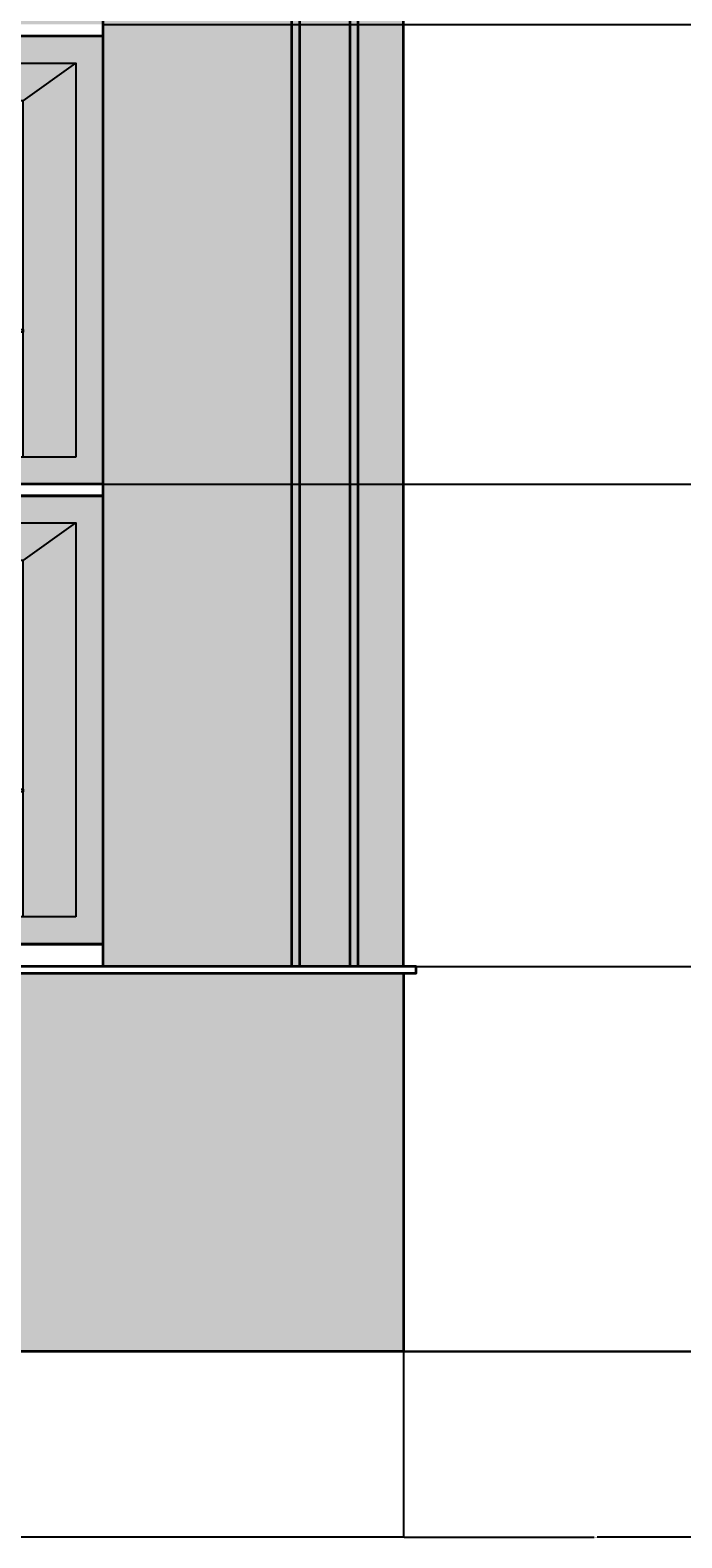
# Model space of a CAD drawing. Units: feet. Extents: x 1141 to 2858, y 751 to 1654.
# Tile 4 of 13: x 2096 to 2288, y 751 to 1195. Entities that reach past the tile are written whole.
import ezdxf

# ---------------------------------------------------------------- set-up
doc = ezdxf.new("R2010")
doc.units = ezdxf.units.FT
for name, color, linetype, lineweight in [('A-ANNO-DIMS', 2, 'Continuous', 18), ('A-ELEV', 7, 'Continuous', 35), ('A-ELEV-PATT', 8, 'Continuous', 13), ('A-GLAZ', 4, 'Continuous', 25)]:
    doc.layers.add(name, color=color, linetype=linetype, lineweight=lineweight)
doc.styles.get("Standard").update_dxf_attribs({"font": 'arial.ttf'})
doc.dimstyles.get("Standard").update_dxf_attribs({"dimtxt": 0.18, "dimasz": 0.18, "dimexe": 0.18, "dimexo": 0.0625, "dimgap": 0.09, "dimtad": 0, "dimtih": 1, "dimtoh": 1, "dimdec": 1, "dimzin": 0, "dimdsep": 46, "dimlunit": 3, "dimtxsty": 'Standard', "dimcen": 0.09, "dimadec": 0, "dimazin": 0, "dimtfac": 1, "dimtdec": 1, "dimtofl": 0, "dimtmove": 0, "dimatfit": 3, "dimfxl": 1, "dimtolj": 1, "dimtzin": 0, "dimarcsym": 0})

# ---------------------------------------------------------------- blocks, each defined once
blk = doc.blocks.new('WIN-SIDE-A')
blk.add_line((63.09, 104.94), (78.57, 116.03))
blk.add_line((63.09, 104.94), (78.57, 116.03))
for points in [[(78.57, 0), (0, 0), (0, 116.03), (78.57, 116.03)], [(78.57, 0), (0, 0), (0, 116.03), (78.57, 116.03)], [(31.54, 104.94), (32.46, 104.94), (32.46, 0), (31.54, 0)], [(0, 37.61), (63.09, 37.61), (63.09, 36.79), (0, 36.79)]]:
    blk.add_lwpolyline(points, close=True)
for points in [[(63.09, 0), (63.09, 104.94), (0, 104.94)], [(63.09, 0), (63.09, 104.94), (0, 104.94)], [(31.54, 37.61), (31.54, 104.94), (32.46, 104.94), (32.46, 37.61)], [(31.54, 36.79), (0, 36.79), (0, 37.61), (31.54, 37.61)], [(32.46, 36.79), (32.46, 0), (31.54, 0), (31.54, 36.79)], [(32.46, 37.61), (63.09, 37.61), (63.09, 36.79), (32.46, 36.79)]]:
    blk.add_lwpolyline(points)
blk = doc.blocks.new('*D22')
at = {"layer": 'A-ANNO-DIMS', "color": 0, "lineweight": -2, "transparency": 16777216}
for p, q in [((1726.03, 805.84), (1726.03, 751.07)), ((2206.03, 805.84), (2206.03, 751.07)), ((1726.21, 751.25), (1965.74, 751.25)), ((2205.85, 751.25), (1966.32, 751.25))]:
    blk.add_line(p, q, dxfattribs=at)
at = {"layer": 'A-ANNO-DIMS', "color": 0, "transparency": 16777216}
for points in [[(1726.21, 751.28), (1726.21, 751.22), (1726.03, 751.25)], [(2205.85, 751.28), (2205.85, 751.22), (2206.03, 751.25)]]:
    blk.add_solid(points, dxfattribs=at)
at = {"layer": 'Defpoints', "color": 0, "transparency": 16777216}
for p in [(1726.03, 805.9), (2206.03, 805.9), (2206.03, 751.25)]:
    blk.add_point(p, dxfattribs=at)
at = {"layer": 'A-ANNO-DIMS', "color": 0, "transparency": 16777216, "insert": (1966.03, 751.25), "char_height": 0.18, "attachment_point": 5}
blk.add_mtext('\\A1;480', dxfattribs=at)
blk = doc.blocks.new('*D23')
at = {"layer": 'A-ANNO-DIMS', "color": 0, "lineweight": -2, "transparency": 16777216}
for p, q in [((2206.03, 805.84), (2206.03, 751.07)), ((2319.3, 805.84), (2319.3, 751.07)), ((2206.21, 751.25), (2262.21, 751.25)), ((2319.12, 751.25), (2263.12, 751.25))]:
    blk.add_line(p, q, dxfattribs=at)
at = {"layer": 'A-ANNO-DIMS', "color": 0, "transparency": 16777216}
for points in [[(2206.21, 751.28), (2206.21, 751.22), (2206.03, 751.25)], [(2319.12, 751.28), (2319.12, 751.22), (2319.3, 751.25)]]:
    blk.add_solid(points, dxfattribs=at)
at = {"layer": 'Defpoints', "color": 0, "transparency": 16777216}
for p in [(2206.03, 805.9), (2319.3, 805.9), (2319.3, 751.25)]:
    blk.add_point(p, dxfattribs=at)
at = {"layer": 'A-ANNO-DIMS', "color": 0, "transparency": 16777216, "insert": (2262.67, 751.25), "char_height": 0.18, "attachment_point": 5}
blk.add_mtext('\\A1;113.27', dxfattribs=at)
blk = doc.blocks.new('*D29')
at = {"layer": 'A-ANNO-DIMS', "color": 0, "lineweight": -2, "transparency": 16777216}
for p, q in [((2206.09, 919.34), (2857.83, 919.34)), ((2857.65, 919.16), (2857.65, 862.8)), ((2857.65, 806.08), (2857.65, 862.44)), ((2206.09, 805.9), (2857.83, 805.9))]:
    blk.add_line(p, q, dxfattribs=at)
at = {"layer": 'A-ANNO-DIMS', "color": 0, "transparency": 16777216}
for points in [[(2857.62, 919.16), (2857.68, 919.16), (2857.65, 919.34)], [(2857.62, 806.08), (2857.68, 806.08), (2857.65, 805.9)]]:
    blk.add_solid(points, dxfattribs=at)
at = {"layer": 'Defpoints', "color": 0, "transparency": 16777216}
for p in [(2206.03, 919.34), (2857.65, 919.34), (2206.03, 805.9)]:
    blk.add_point(p, dxfattribs=at)
at = {"layer": 'A-ANNO-DIMS', "color": 0, "transparency": 16777216, "insert": (2857.65, 862.62), "char_height": 0.18, "attachment_point": 5}
blk.add_mtext('\\A1;113.44', dxfattribs=at)
blk = doc.blocks.new('*D30')
at = {"layer": 'A-ANNO-DIMS', "color": 0, "lineweight": -2, "transparency": 16777216}
for p, q in [((2117.47, 1061.29), (2857.83, 1061.29)), ((2857.65, 1061.11), (2857.65, 990.5)), ((2857.65, 919.52), (2857.65, 990.13)), ((2117.47, 919.34), (2857.83, 919.34))]:
    blk.add_line(p, q, dxfattribs=at)
at = {"layer": 'A-ANNO-DIMS', "color": 0, "transparency": 16777216}
for points in [[(2857.62, 1061.11), (2857.68, 1061.11), (2857.65, 1061.29)], [(2857.62, 919.52), (2857.68, 919.52), (2857.65, 919.34)]]:
    blk.add_solid(points, dxfattribs=at)
at = {"layer": 'Defpoints', "color": 0, "transparency": 16777216}
for p in [(2117.41, 1061.29), (2857.65, 1061.29), (2117.41, 919.34)]:
    blk.add_point(p, dxfattribs=at)
at = {"layer": 'A-ANNO-DIMS', "color": 0, "transparency": 16777216, "insert": (2857.65, 990.31), "char_height": 0.18, "attachment_point": 5}
blk.add_mtext('\\A1;141.95', dxfattribs=at)
blk = doc.blocks.new('*D31')
at = {"layer": 'A-ANNO-DIMS', "color": 0, "lineweight": -2, "transparency": 16777216}
for p, q in [((2117.47, 1196.68), (2857.83, 1196.68)), ((2857.65, 1196.5), (2857.65, 1129.16)), ((2857.65, 1061.47), (2857.65, 1128.8)), ((2117.47, 1061.29), (2857.83, 1061.29))]:
    blk.add_line(p, q, dxfattribs=at)
at = {"layer": 'A-ANNO-DIMS', "color": 0, "transparency": 16777216}
for points in [[(2857.62, 1196.5), (2857.68, 1196.5), (2857.65, 1196.68)], [(2857.62, 1061.47), (2857.68, 1061.47), (2857.65, 1061.29)]]:
    blk.add_solid(points, dxfattribs=at)
at = {"layer": 'Defpoints', "color": 0, "transparency": 16777216}
for p in [(2117.41, 1196.68), (2857.65, 1196.68), (2117.41, 1061.29)]:
    blk.add_point(p, dxfattribs=at)
at = {"layer": 'A-ANNO-DIMS', "color": 0, "transparency": 16777216, "insert": (2857.65, 1128.98), "char_height": 0.18, "attachment_point": 5}
blk.add_mtext('\\A1;135.4', dxfattribs=at)
blk = doc.blocks.new('*D39')
at = {"layer": 'A-ANNO-DIMS', "color": 0, "lineweight": -2, "transparency": 16777216}
for p, q in [((2319.24, 1599.45), (1668.14, 1599.45)), ((1668.32, 1599.27), (1668.32, 1202.86)), ((1668.32, 806.08), (1668.32, 1202.49)), ((2319.24, 805.9), (1668.14, 805.9))]:
    blk.add_line(p, q, dxfattribs=at)
at = {"layer": 'A-ANNO-DIMS', "color": 0, "transparency": 16777216}
for points in [[(1668.29, 1599.27), (1668.35, 1599.27), (1668.32, 1599.45)], [(1668.29, 806.08), (1668.35, 806.08), (1668.32, 805.9)]]:
    blk.add_solid(points, dxfattribs=at)
at = {"layer": 'Defpoints', "color": 0, "transparency": 16777216}
for p in [(1668.32, 1599.45), (2319.3, 1599.45), (2319.3, 805.9)]:
    blk.add_point(p, dxfattribs=at)
at = {"layer": 'A-ANNO-DIMS', "color": 0, "transparency": 16777216, "insert": (1668.32, 1202.68), "char_height": 0.18, "attachment_point": 5}
blk.add_mtext('\\A1;793.6', dxfattribs=at)

msp = doc.modelspace()

# ---------------------------------------------------------------- hatches: boundary and pattern name
at = {"layer": 'A-ELEV-PATT'}
h = msp.add_hatch(color=256, dxfattribs=at)
h.dxf.hatch_style = 1
h.paths.add_polyline_path([(2206.032, 1599.4527), (2192.689, 1599.4527), (2192.689, 919.339), (2206.032, 919.339)])
h.paths.add_polyline_path([(2190.2416, 1599.4527), (2175.463, 1599.4527), (2175.463, 919.339), (2190.2416, 919.339)])
h.paths.add_polyline_path([(2173.0156, 1599.4527), (2117.407, 1599.4527), (2117.407, 919.339), (2173.0156, 919.339)])
h.paths.add_polyline_path([(2022.8666, 1057.9008), (1726.032, 1057.9008), (1726.032, 925.9008), (2022.8666, 925.9008)])
h.paths.add_polyline_path([(1737.6123, 937.4811), (1737.6123, 1046.3205), (2011.2863, 1046.3205), (2011.2863, 937.4811)], flags=16)
h.paths.add_polyline_path([(1754.2423, 946.7736), (1754.2423, 1033.2183), (2004.2323, 1033.2183), (2004.2323, 946.7736), (2004.3069, 946.6754), (1906.0824, 946.6754)], flags=0)
h.paths.add_polyline_path([(1900.5421, 946.7736), (1857.5566, 946.7736), (1857.5566, 1033.2183), (1900.5421, 1033.2183)], flags=0)
h.paths.add_polyline_path([(1910.8368, 951.4297), (1910.8368, 1022.7957), (1999.478, 1022.7957), (1999.478, 951.4297)], flags=0)
h.paths.add_polyline_path([(1930.8039, 951.4297), (1930.8039, 1022.7957), (1932.373, 1022.7957), (1932.373, 951.4297)], flags=0)
h.paths.add_polyline_path([(1851.6414, 946.7736), (1826.5664, 946.7736), (1826.5664, 967.8234), (1793.4402, 967.8234), (1793.4402, 946.7736), (1790.4043, 946.7736), (1790.4043, 967.8234), (1754.2423, 967.8234), (1754.2423, 970.4796), (1790.4043, 970.4796), (1790.4043, 1033.2183), (1793.4402, 1033.2183), (1793.4402, 970.4796), (1826.5664, 970.4796), (1826.5664, 1033.2183), (1851.6414, 1033.2183)], flags=0)
h.paths.add_polyline_path([(1954.3728, 951.4297), (1954.3728, 1022.7957), (1955.9419, 1022.7957), (1955.9419, 951.4297)], flags=0)
h.paths.add_polyline_path([(1977.7327, 951.4297), (1977.7327, 1022.7957), (1979.3018, 1022.7957), (1979.3018, 951.4297)], flags=0)
h.paths.add_polyline_path([(2022.8666, 1193.2888), (1726.032, 1193.2888), (1726.032, 1061.2888), (2022.8666, 1061.2888)])
h.paths.add_polyline_path([(1737.6123, 1072.869), (1737.6123, 1181.7085), (2011.2863, 1181.7085), (2011.2863, 1072.869)], flags=16)
h.paths.add_polyline_path([(1754.2423, 1082.1616), (1754.2423, 1168.6063), (2004.2323, 1168.6063), (2004.2323, 1082.1616), (2004.3069, 1082.0634), (1906.0824, 1082.0634)], flags=0)
h.paths.add_polyline_path([(1900.5421, 1082.1616), (1857.5566, 1082.1616), (1857.5566, 1168.6063), (1900.5421, 1168.6063)], flags=0)
h.paths.add_polyline_path([(1910.8368, 1086.8177), (1910.8368, 1158.1837), (1999.478, 1158.1837), (1999.478, 1086.8177)], flags=0)
h.paths.add_polyline_path([(1930.8039, 1086.8177), (1930.8039, 1158.1837), (1932.373, 1158.1837), (1932.373, 1086.8177)], flags=0)
h.paths.add_polyline_path([(1851.6414, 1082.1616), (1826.5664, 1082.1616), (1826.5664, 1103.2114), (1793.4402, 1103.2114), (1793.4402, 1082.1616), (1790.4043, 1082.1616), (1790.4043, 1103.2114), (1754.2423, 1103.2114), (1754.2423, 1105.8676), (1790.4043, 1105.8676), (1790.4043, 1168.6063), (1793.4402, 1168.6063), (1793.4402, 1105.8676), (1826.5664, 1105.8676), (1826.5664, 1168.6063), (1851.6414, 1168.6063)], flags=0)
h.paths.add_polyline_path([(1954.3728, 1086.8177), (1954.3728, 1158.1837), (1955.9419, 1158.1837), (1955.9419, 1086.8177)], flags=0)
h.paths.add_polyline_path([(1977.7327, 1086.8177), (1977.7327, 1158.1837), (1979.3018, 1158.1837), (1979.3018, 1086.8177)], flags=0)
h.paths.add_polyline_path([(2022.8666, 1599.4527), (1726.032, 1599.4527), (1726.032, 1467.4527), (2022.8666, 1467.4527)])
h.paths.add_polyline_path([(2011.2863, 1479.033), (1737.6123, 1479.033), (1737.6123, 1587.8725), (2011.2863, 1587.8725)], flags=16)
h.paths.add_polyline_path([(2004.2323, 1488.3255), (1754.2423, 1488.3255), (1754.2423, 1574.7702), (2004.2323, 1574.7702)], flags=0)
h.paths.add_polyline_path([(1829.1345, 1544.6458), (1914.1177, 1544.6458), (1914.1177, 1539.5463), (1830.9097, 1539.5463), (1831.6817, 1537.3286), (1914.1177, 1537.3286), (1914.1177, 1532.2291), (1833.4569, 1532.2291), (1834.229, 1530.0113), (1914.1177, 1530.0113), (1914.1177, 1524.9118), (1836.0042, 1524.9118), (1836.7762, 1522.694), (1914.1177, 1522.694), (1914.1177, 1517.5946), (1838.5514, 1517.5946), (1839.3235, 1515.3768), (1914.1177, 1515.3768), (1914.1177, 1510.2773), (1841.0987, 1510.2773), (1841.8707, 1508.0595), (1914.1177, 1508.0595), (1914.1177, 1502.9601), (1843.6459, 1502.9601), (1844.4179, 1500.7423), (1914.1177, 1500.7423), (1914.1177, 1495.6428), (1846.1931, 1495.6428), (1846.9652, 1493.425), (1914.1177, 1493.425), (1914.1177, 1488.3255), (1848.6593, 1488.3255), (1848.6593, 1488.5583)], flags=0)
h.paths.add_polyline_path([(2117.407, 1464.0647), (1820.5724, 1464.0647), (1820.5724, 1332.0647), (2117.407, 1332.0647)])
h.paths.add_polyline_path([(2105.8267, 1452.4845), (2105.8267, 1343.645), (1832.1527, 1343.645), (1832.1527, 1452.4845)], flags=16)
h.paths.add_polyline_path([(2089.1967, 1439.3822), (2089.1967, 1352.9376), (1937.3566, 1352.9376), (1937.3566, 1352.8393), (1839.1321, 1352.8393), (1839.2067, 1352.9376), (1839.2067, 1439.3822), (1937.3566, 1439.3822)], flags=0)
h.paths.add_polyline_path([(2016.8727, 1439.3822), (2016.8727, 1376.6436), (2049.9988, 1376.6436), (2049.9988, 1439.3822), (2053.0347, 1439.3822), (2053.0347, 1376.6436), (2089.1967, 1376.6436), (2089.1967, 1373.9873), (2053.0347, 1373.9873), (2053.0347, 1352.9376), (2049.9988, 1352.9376), (2049.9988, 1373.9873), (2016.8727, 1373.9873), (2016.8727, 1352.9376), (1991.7976, 1352.9376), (1991.7976, 1439.3822)], flags=0)
h.paths.add_polyline_path([(1985.8824, 1439.3822), (1985.8824, 1352.9376), (1942.8969, 1352.9376), (1942.8969, 1439.3822)], flags=0)
h.paths.add_polyline_path([(1932.6022, 1428.9596), (1932.6022, 1357.5937), (1843.961, 1357.5937), (1843.961, 1428.9596)], flags=0)
h.paths.add_polyline_path([(1912.6351, 1428.9596), (1912.6351, 1357.5937), (1911.066, 1357.5937), (1911.066, 1428.9596)], flags=0)
h.paths.add_polyline_path([(1889.0662, 1428.9596), (1889.0662, 1357.5937), (1887.4971, 1357.5937), (1887.4971, 1428.9596)], flags=0)
h.paths.add_polyline_path([(1865.7063, 1428.9596), (1865.7063, 1357.5937), (1864.1372, 1357.5937), (1864.1372, 1428.9596)], flags=0)
h.paths.add_polyline_path([(2117.407, 1328.6768), (1820.5724, 1328.6768), (1820.5724, 1196.6768), (2117.407, 1196.6768)])
h.paths.add_polyline_path([(2105.8267, 1317.0965), (2105.8267, 1208.257), (1832.1527, 1208.257), (1832.1527, 1317.0965)], flags=16)
h.paths.add_polyline_path([(2089.1967, 1303.9943), (2089.1967, 1217.5496), (1937.3566, 1217.5496), (1937.3566, 1217.4513), (1839.1321, 1217.4513), (1839.2067, 1217.5496), (1839.2067, 1303.9943), (1937.3566, 1303.9943)], flags=0)
h.paths.add_polyline_path([(2016.8727, 1303.9943), (2016.8727, 1241.2556), (2049.9988, 1241.2556), (2049.9988, 1303.9943), (2053.0347, 1303.9943), (2053.0347, 1241.2556), (2089.1967, 1241.2556), (2089.1967, 1238.5993), (2053.0347, 1238.5993), (2053.0347, 1217.5496), (2049.9988, 1217.5496), (2049.9988, 1238.5993), (2016.8727, 1238.5993), (2016.8727, 1217.5496), (1991.7976, 1217.5496), (1991.7976, 1303.9943)], flags=0)
h.paths.add_polyline_path([(1985.8824, 1303.9943), (1985.8824, 1217.5496), (1942.8969, 1217.5496), (1942.8969, 1303.9943)], flags=0)
h.paths.add_polyline_path([(1932.6022, 1293.5716), (1932.6022, 1222.2057), (1843.961, 1222.2057), (1843.961, 1293.5716)], flags=0)
h.paths.add_polyline_path([(1912.6351, 1293.5716), (1912.6351, 1222.2057), (1911.066, 1222.2057), (1911.066, 1293.5716)], flags=0)
h.paths.add_polyline_path([(1889.0662, 1293.5716), (1889.0662, 1222.2057), (1887.4971, 1222.2057), (1887.4971, 1293.5716)], flags=0)
h.paths.add_polyline_path([(1865.7063, 1293.5716), (1865.7063, 1222.2057), (1864.1372, 1222.2057), (1864.1372, 1293.5716)], flags=0)
h.paths.add_polyline_path([(2206.032, 917.3598), (2027.2589, 917.3598), (2027.2589, 805.9008), (2206.032, 805.9008)])
h.paths.add_polyline_path([(1852.1771, 917.3598), (1726.032, 917.3598), (1726.032, 805.9008), (1852.1771, 805.9008)])
h.paths.add_polyline_path([(2063.3101, 1580.3829), (2093.938, 1580.3829), (2093.938, 1513.0494), (2063.3101, 1513.0494)])
h.paths.add_polyline_path([(2063.3101, 1580.3829), (2093.938, 1580.3829), (2093.938, 1513.0494), (2063.3101, 1513.0494)])
h = msp.add_hatch(color=256, dxfattribs=at)
h.dxf.hatch_style = 1
h.paths.add_polyline_path([(2011.2863, 1587.8725), (1737.6123, 1587.8725), (1754.2423, 1574.7702), (2004.2323, 1574.7702)])
h.paths.add_polyline_path([(1754.2423, 1574.7702), (1737.6123, 1587.8725), (1737.6123, 1479.033), (1754.2423, 1488.3255)])
h.paths.add_polyline_path([(2011.2863, 1587.8725), (2004.2323, 1574.7702), (2004.2323, 1488.3255), (2011.2863, 1479.033)])
h.paths.add_polyline_path([(2004.2323, 1488.3255), (1754.2423, 1488.3255), (1737.6123, 1479.033), (2011.2863, 1479.033)])
h.paths.add_polyline_path([(2105.8267, 1452.4845), (1832.1527, 1452.4845), (1839.2067, 1439.3822), (1937.3566, 1439.3822), (2089.1967, 1439.3822)])
h.paths.add_polyline_path([(1839.2067, 1439.3822), (1832.1527, 1452.4845), (1832.1527, 1343.645), (1839.2067, 1352.9376)])
h.paths.add_polyline_path([(2105.8267, 1452.4845), (2089.1967, 1439.3822), (2089.1967, 1352.9376), (2105.8267, 1343.645)])
h.paths.add_polyline_path([(2089.1967, 1352.9376), (1937.3566, 1352.9376), (1937.3566, 1352.8393), (1839.1321, 1352.8393), (1832.1527, 1343.645), (2105.8267, 1343.645)])
h.paths.add_polyline_path([(1942.8969, 1439.3822), (1937.3566, 1439.3822), (1937.3566, 1352.9376), (1942.8969, 1352.9376)])
h.paths.add_polyline_path([(1991.7976, 1439.3822), (1985.8824, 1439.3822), (1985.8824, 1352.9376), (1991.7976, 1352.9376)])
h.paths.add_polyline_path([(2109.4211, 1591.4669), (2030.8524, 1591.4669), (2030.8524, 1580.3829), (2093.938, 1580.3829)])
h.paths.add_polyline_path([(2109.4211, 1591.4669), (2093.938, 1580.3829), (2093.938, 1475.4386), (2109.4211, 1475.4386)])
h.paths.add_polyline_path([(1991.7976, 1303.9943), (1985.8824, 1303.9943), (1985.8824, 1217.5496), (1991.7976, 1217.5496)])
h.paths.add_polyline_path([(1942.8969, 1303.9943), (1937.3566, 1303.9943), (1937.3566, 1217.5496), (1942.8969, 1217.5496)])
h.paths.add_polyline_path([(2105.8267, 1317.0965), (1832.1527, 1317.0965), (1839.2067, 1303.9943), (1937.3566, 1303.9943), (2089.1967, 1303.9943)])
h.paths.add_polyline_path([(1839.2067, 1303.9943), (1832.1527, 1317.0965), (1832.1527, 1208.257), (1839.2067, 1217.5496)])
h.paths.add_polyline_path([(2089.1967, 1217.5496), (1937.3566, 1217.5496), (1937.3566, 1217.4513), (1839.1321, 1217.4513), (1832.1527, 1208.257), (2105.8267, 1208.257)])
h.paths.add_polyline_path([(2105.8267, 1317.0965), (2089.1967, 1303.9943), (2089.1967, 1217.5496), (2105.8267, 1208.257)])
h.paths.add_polyline_path([(1754.2423, 1168.6063), (1737.6123, 1181.7085), (1737.6123, 1072.869), (1754.2423, 1082.1616)])
h.paths.add_polyline_path([(2011.2863, 1181.7085), (1737.6123, 1181.7085), (1754.2423, 1168.6063), (2004.2323, 1168.6063)])
h.paths.add_polyline_path([(2011.2863, 1181.7085), (2004.2323, 1168.6063), (2004.2323, 1082.1616), (2011.2863, 1072.869)])
h.paths.add_polyline_path([(2004.3069, 1082.0634), (1906.0824, 1082.0634), (1754.2423, 1082.1616), (1737.6123, 1072.869), (2011.2863, 1072.869)])
h.paths.add_polyline_path([(1906.0824, 1168.6063), (1900.5421, 1168.6063), (1900.5421, 1082.1616), (1906.0824, 1082.1616)])
h.paths.add_polyline_path([(1857.5566, 1168.6063), (1851.6414, 1168.6063), (1851.6414, 1082.1616), (1857.5566, 1082.1616)])
h.paths.add_polyline_path([(1906.0824, 1033.2183), (1900.5421, 1033.2183), (1900.5421, 946.7736), (1906.0824, 946.7736)])
h.paths.add_polyline_path([(1857.5566, 1033.2183), (1851.6414, 1033.2183), (1851.6414, 946.7736), (1857.5566, 946.7736)])
h.paths.add_polyline_path([(1754.2423, 1033.2183), (1737.6123, 1046.3205), (1737.6123, 937.4811), (1754.2423, 946.7736)])
h.paths.add_polyline_path([(2011.2863, 1046.3205), (1737.6123, 1046.3205), (1754.2423, 1033.2183), (2004.2323, 1033.2183)])
h.paths.add_polyline_path([(2011.2863, 1046.3205), (2004.2323, 1033.2183), (2004.2323, 946.7736), (2011.2863, 937.4811)])
h.paths.add_polyline_path([(2004.3069, 946.6754), (1906.0824, 946.6754), (1754.2423, 946.7736), (1737.6123, 937.4811), (2011.2863, 937.4811)])
h.paths.add_polyline_path([(2175.463, 1599.4527), (2173.0156, 1599.4527), (2173.0156, 919.339), (2175.463, 919.339)])
h = msp.add_hatch(color=256, dxfattribs=at)
h.dxf.hatch_style = 1
h.paths.add_polyline_path([(2192.689, 1599.4527), (2190.2416, 1599.4527), (2190.2416, 919.339), (2192.689, 919.339)])
h = msp.add_hatch(color=256, dxfattribs=at)
h.dxf.hatch_style = 1
h.paths.add_polyline_path([(1812.5866, 1456.0789), (1734.0179, 1456.0789), (1749.501, 1444.9949), (1812.5866, 1444.9949)], flags=0)
h.paths.add_polyline_path([(1820.5724, 1464.0647), (1726.032, 1464.0647), (1726.032, 1332.0647), (1820.5724, 1332.0647)])
h.paths.add_polyline_path([(1734.0179, 1456.0789), (1812.5866, 1456.0789), (1812.5866, 1340.0506), (1734.0179, 1340.0506)], flags=16)
h.paths.add_polyline_path([(1749.501, 1444.9949), (1781.0438, 1444.9949), (1781.0438, 1377.6615), (1812.5866, 1377.6615), (1812.5866, 1376.842), (1781.0438, 1376.842), (1781.0438, 1340.0506), (1780.1289, 1340.0506), (1780.1289, 1376.842), (1749.501, 1376.842), (1749.501, 1377.6615)], flags=0)
h.paths.add_polyline_path([(1749.501, 1444.9949), (1734.0179, 1456.0789), (1734.0179, 1340.0506), (1749.501, 1340.0506)], flags=0)
h.paths.add_polyline_path([(1820.5724, 1328.6768), (1726.032, 1328.6768), (1726.032, 1196.6768), (1820.5724, 1196.6768)])
h.paths.add_polyline_path([(1734.0179, 1320.6909), (1812.5866, 1320.6909), (1812.5866, 1204.6626), (1734.0179, 1204.6626)], flags=16)
h.paths.add_polyline_path([(1749.501, 1309.6069), (1781.0438, 1309.6069), (1781.0438, 1242.2735), (1812.5866, 1242.2735), (1812.5866, 1241.454), (1781.0438, 1241.454), (1781.0438, 1204.6626), (1780.1289, 1204.6626), (1780.1289, 1241.454), (1749.501, 1241.454), (1749.501, 1242.2735)], flags=0)
h.paths.add_polyline_path([(1749.501, 1309.6069), (1734.0179, 1320.6909), (1734.0179, 1204.6626), (1749.501, 1204.6626)], flags=0)
h.paths.add_polyline_path([(2117.407, 1193.2888), (2022.8666, 1193.2888), (2022.8666, 1061.2888), (2117.407, 1061.2888)])
h.paths.add_polyline_path([(2109.4211, 1185.3029), (2109.4211, 1069.2747), (2030.8524, 1069.2747), (2030.8524, 1185.3029)], flags=16)
h.paths.add_polyline_path([(2093.938, 1174.219), (2093.938, 1106.066), (2063.3101, 1106.066), (2063.3101, 1069.2747), (2062.3952, 1069.2747), (2062.3952, 1106.066), (2030.8524, 1106.066), (2030.8524, 1106.8855), (2062.3952, 1106.8855), (2062.3952, 1174.219), (2063.3101, 1174.219)], flags=0)
h.paths.add_polyline_path([(2702.6903, 1049.9149), (2624.1217, 1049.9149), (2624.1217, 1038.831), (2687.2072, 1038.831), (2687.2072, 933.8867), (2702.6903, 933.8867)], flags=0)
h.paths.add_polyline_path([(2109.4211, 1049.9149), (2093.938, 1038.831), (2093.938, 933.8867), (2109.4211, 933.8867)])
h.paths.add_polyline_path([(2109.4211, 1049.9149), (2030.8524, 1049.9149), (2030.8524, 1038.831), (2093.938, 1038.831)])
h = msp.add_hatch(color=256, dxfattribs=at)
h.dxf.hatch_style = 1
h.paths.add_polyline_path([(1219.3173, 1456.0789), (1140.7487, 1456.0789), (1156.2318, 1444.9949), (1219.3173, 1444.9949)], flags=0)
h.paths.add_polyline_path([(1156.2318, 1444.9949), (1140.7487, 1456.0789), (1140.7487, 1340.0506), (1156.2318, 1340.0506)], flags=0)
h.paths.add_polyline_path([(1156.2318, 1309.6069), (1187.7746, 1309.6069), (1187.7746, 1242.2735), (1219.3173, 1242.2735), (1219.3173, 1241.454), (1187.7746, 1241.454), (1187.7746, 1204.6626), (1186.8597, 1204.6626), (1186.8597, 1241.454), (1156.2318, 1241.454), (1156.2318, 1242.2735)], flags=0)
h.paths.add_polyline_path([(2109.4211, 1049.9149), (2030.8524, 1049.9149), (2030.8524, 1038.831), (2093.938, 1038.831), (2093.938, 933.8867), (2109.4211, 933.8867)], flags=0)
h.paths.add_polyline_path([(2109.4211, 1185.3029), (2030.8524, 1185.3029), (2030.8524, 1174.219), (2093.938, 1174.219), (2093.938, 1069.2747), (2109.4211, 1069.2747)])
h.paths.add_polyline_path([(1812.5866, 1320.6909), (1734.0179, 1320.6909), (1749.501, 1309.6069), (1812.5866, 1309.6069)])
h.paths.add_polyline_path([(1749.501, 1309.6069), (1734.0179, 1320.6909), (1734.0179, 1204.6626), (1749.501, 1204.6626)])
h.paths.add_polyline_path([(1812.5866, 1456.0789), (1734.0179, 1456.0789), (1749.501, 1444.9949), (1812.5866, 1444.9949)])
h.paths.add_polyline_path([(2117.407, 1057.9008), (2022.8666, 1057.9008), (2022.8666, 925.9008), (2117.407, 925.9008)])
h.paths.add_polyline_path([(2030.8524, 933.8867), (2030.8524, 1049.9149), (2109.4211, 1049.9149), (2109.4211, 933.8867)], flags=16)
h.paths.add_polyline_path([(2062.3952, 933.8867), (2062.3952, 970.6781), (2030.8524, 970.6781), (2030.8524, 971.4975), (2062.3952, 971.4975), (2062.3952, 1038.831), (2063.3101, 1038.831), (2093.938, 1038.831), (2093.938, 970.6781), (2063.3101, 970.6781), (2063.3101, 933.8867)], flags=0)

# ---------------------------------------------------------------- linework, layer by layer
at = {"layer": 'A-ELEV'}
for p, q in [((2117.407, 1057.9008), (1726.032, 1057.9008)), ((2117.407, 1057.9008), (1726.032, 1057.9008)), ((1726.032, 925.9008), (2117.407, 925.9008)), ((1726.032, 925.9008), (2117.407, 925.9008))]:
    msp.add_line(p, q, dxfattribs=at)
for points in [[(2206.032, 919.339), (2206.032, 1599.4527), (2117.407, 1599.4527), (2117.407, 919.339)], [(2206.032, 919.339), (2206.032, 1599.4527), (2117.407, 1599.4527), (2117.407, 919.339)], [(2175.463, 919.339), (2175.463, 1599.4527), (2173.0156, 1599.4527), (2173.0156, 919.339)], [(2192.689, 919.339), (2192.689, 1599.4527), (2190.2416, 1599.4527), (2190.2416, 919.339)], [(2192.689, 919.339), (2192.689, 1599.4527), (2190.2416, 1599.4527), (2190.2416, 919.339)], [(2192.689, 919.339), (2192.689, 1599.4527), (2190.2416, 1599.4527), (2190.2416, 919.339)], [(2117.407, 917.3598), (2206.032, 917.3598)], [(2117.407, 917.3598), (2206.032, 917.3598)], [(2173.0156, 917.3598), (2175.463, 917.3598)], [(2173.0156, 917.3598), (2175.463, 917.3598)], [(2190.2416, 917.3598), (2192.689, 917.3598)], [(2190.2416, 917.3598), (2192.689, 917.3598)]]:
    msp.add_lwpolyline(points, dxfattribs=at)
for points in [[(2117.407, 1061.2888), (2022.8666, 1061.2888), (2022.8666, 1193.2888), (2117.407, 1193.2888)], [(2117.407, 1061.2888), (2022.8666, 1061.2888), (2022.8666, 1193.2888), (2117.407, 1193.2888)], [(2117.407, 925.9008), (2022.8666, 925.9008), (2022.8666, 1057.9008), (2117.407, 1057.9008)], [(2117.407, 925.9008), (2022.8666, 925.9008), (2022.8666, 1057.9008), (2117.407, 1057.9008)], [(2023.7788, 917.3598), (2209.7297, 917.3598), (2209.7297, 919.339), (2023.7788, 919.339)], [(2023.7788, 917.3598), (2209.7297, 917.3598), (2209.7297, 919.339), (2023.7788, 919.339)], [(2206.032, 805.9008), (2027.2589, 805.9008), (2027.2589, 917.3598), (2206.032, 917.3598)], [(2206.032, 805.9008), (2027.2589, 805.9008), (2027.2589, 917.3598), (2206.032, 917.3598)]]:
    msp.add_lwpolyline(points, close=True, dxfattribs=at)

# ---------------------------------------------------------------- block references
at = {"layer": 'A-GLAZ'}
for p in [(2030.852, 1069.2751), (2030.852, 933.8871)]:
    msp.add_blockref('WIN-SIDE-A', p, dxfattribs=at)

# ---------------------------------------------------------------- dimensions: what is measured, and where the dimension line sits
at = {"layer": 'A-ANNO-DIMS'}
for base, p1, p2, override, picture, middle in [((1668.3207, 1599.4527), (2319.3013, 805.9008), (2319.3013, 1599.4527), {"dimdec": 1, "dimlfac": 1, "dimrnd": 0, "dimzin": 0, "dimdsep": 46, "dimlunit": 2}, '*D39', (1668.3207, 1202.6768)), ((2857.6489, 1196.6768), (2117.407, 1061.2888), (2117.407, 1196.6768), {"dimdec": 1, "dimlfac": 1, "dimrnd": 0, "dimzin": 0, "dimdsep": 46, "dimlunit": 2}, '*D31', (2857.6489, 1128.9828)), ((2857.6489, 1061.2888), (2117.407, 919.339), (2117.407, 1061.2888), {"dimdec": 2, "dimlfac": 1, "dimrnd": 0, "dimzin": 0, "dimdsep": 46, "dimlunit": 2}, '*D30', (2857.6489, 990.3139)), ((2857.6489, 919.339), (2206.032, 805.9008), (2206.032, 919.339), {"dimdec": 2, "dimlfac": 1, "dimrnd": 0, "dimzin": 0, "dimdsep": 46, "dimlunit": 2}, '*D29', (2857.6489, 862.6199))]:
    dim = msp.add_linear_dim(base=base, p1=p1, p2=p2, angle=90, dimstyle='Standard', override=override, dxfattribs=at)
    dim.commit()
    dim.dimension.update_dxf_attribs({"geometry": picture, "text_midpoint": middle})
for base, p1, p2, override, picture, middle in [((2206.032, 751.2508), (1726.032, 805.9008), (2206.032, 805.9008), {"dimdec": 0, "dimlfac": 1, "dimrnd": 0, "dimzin": 0, "dimdsep": 46, "dimlunit": 2}, '*D22', (1966.032, 751.2508)), ((2319.3013, 751.2508), (2206.032, 805.9008), (2319.3013, 805.9008), {"dimdec": 2, "dimlfac": 1, "dimrnd": 0, "dimzin": 0, "dimdsep": 46, "dimlunit": 2}, '*D23', (2262.6667, 751.2508))]:
    dim = msp.add_linear_dim(base=base, p1=p1, p2=p2, dimstyle='Standard', override=override, dxfattribs=at)
    dim.commit()
    dim.dimension.update_dxf_attribs({"geometry": picture, "text_midpoint": middle})

doc.saveas('drawing.dxf')
